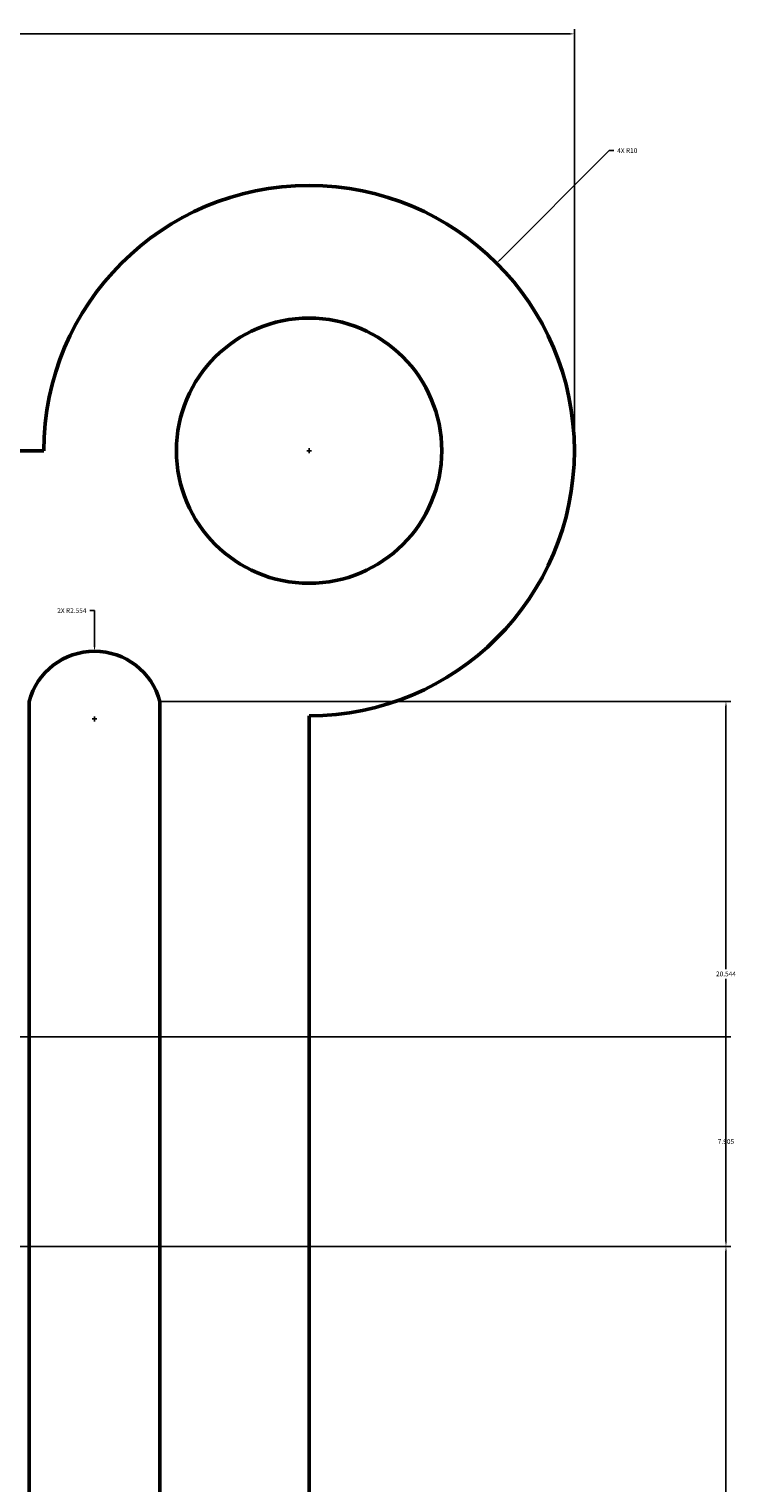
# Model space of a CAD drawing. Units: inches. Extents: x -14 to 108, y -9 to 83.
# Tile 13 of 13: x 82 to 108, y 28 to 83. Entities that reach past the tile are written whole.
import ezdxf

# ---------------------------------------------------------------- set-up
doc = ezdxf.new("R2010")
doc.units = ezdxf.units.IN
doc.header["$MEASUREMENT"] = 0
doc.layers.add('M-DIMS', color=2, linetype='Continuous', lineweight=18)
doc.layers.add('M-OUTL', color=7, linetype='Continuous', lineweight=50)
doc.styles.get("Standard").update_dxf_attribs({"font": 'arial.ttf'})
doc.dimstyles.get("Standard").update_dxf_attribs({"dimtxt": 0.18, "dimasz": 0.18, "dimexe": 0.18, "dimexo": 0.0625, "dimgap": 0.09, "dimtad": 0, "dimtih": 1, "dimtoh": 1, "dimzin": 0, "dimdsep": 46, "dimtxsty": 'Standard', "dimcen": 0.09, "dimadec": 0, "dimazin": 0, "dimtfac": 1, "dimtofl": 0, "dimtmove": 0, "dimatfit": 3, "dimfxl": 1, "dimtolj": 1, "dimtzin": 0, "dimarcsym": 0})

# ---------------------------------------------------------------- blocks, each defined once
blk = doc.blocks.new('SLOT-VERTICAL')
for points in [[(0, 1.021), (0, 40.458)], [(4.933, 40.458), (4.933, 1.021)]]:
    blk.add_lwpolyline(points)
for centre, radius, start, end in [((2.466, 39.797), 2.554, 15, 165), ((2.466, 3.488), 3.489, 225, 315)]:
    blk.add_arc(centre, radius, start, end)
blk = doc.blocks.new('HOLE-D10')
blk.add_circle((5, 5), 5)
blk = doc.blocks.new('*D4')
at = {"layer": 'Defpoints', "color": 0, "transparency": 16777216}
for p in [(102.098, 82.834), (-7.902, 67.119), (102.098, 67.119)]:
    blk.add_point(p, dxfattribs=at)
at = {"layer": 'M-DIMS', "color": 0, "lineweight": -2, "transparency": 16777216}
for p, q in [((-7.902, 67.182), (-7.902, 83.014)), ((-7.722, 82.834), (46.818, 82.834)), ((101.918, 82.834), (47.378, 82.834)), ((102.098, 67.182), (102.098, 83.014))]:
    blk.add_line(p, q, dxfattribs=at)
at = {"layer": 'M-DIMS', "color": 0, "transparency": 16777216}
for points in [[(-7.722, 82.864), (-7.722, 82.804), (-7.902, 82.834)], [(101.918, 82.864), (101.918, 82.804), (102.098, 82.834)]]:
    blk.add_solid(points, dxfattribs=at)
at = {"layer": 'M-DIMS', "color": 0, "transparency": 16777216, "insert": (47.098, 82.834), "char_height": 0.18, "attachment_point": 5}
blk.add_mtext('\\A1;110', dxfattribs=at)
blk = doc.blocks.new('*D11')
at = {"layer": 'Defpoints', "color": 0, "transparency": 16777216}
for p in [(47.098, 37.119), (107.813, 37.119), (86.478, 18.227)]:
    blk.add_point(p, dxfattribs=at)
at = {"layer": 'M-DIMS', "color": 0, "lineweight": -2, "transparency": 16777216}
for p, q in [((47.16, 37.119), (107.993, 37.119)), ((107.813, 36.939), (107.813, 27.855)), ((107.813, 18.407), (107.813, 27.491)), ((86.541, 18.227), (107.993, 18.227))]:
    blk.add_line(p, q, dxfattribs=at)
at = {"layer": 'M-DIMS', "color": 0, "transparency": 16777216}
for points in [[(107.783, 36.939), (107.843, 36.939), (107.813, 37.119)], [(107.783, 18.407), (107.843, 18.407), (107.813, 18.227)]]:
    blk.add_solid(points, dxfattribs=at)
at = {"layer": 'M-DIMS', "color": 0, "transparency": 16777216, "insert": (107.813, 27.673), "char_height": 0.18, "attachment_point": 5}
blk.add_mtext('\\A1;18.892', dxfattribs=at)
blk = doc.blocks.new('*D12')
at = {"layer": 'Defpoints', "color": 0, "transparency": 16777216}
for p in [(86.478, 57.664), (107.813, 57.664), (47.098, 37.119)]:
    blk.add_point(p, dxfattribs=at)
at = {"layer": 'M-DIMS', "color": 0, "lineweight": -2, "transparency": 16777216}
for p, q in [((86.541, 57.664), (107.993, 57.664)), ((107.813, 57.484), (107.813, 47.573)), ((107.813, 37.299), (107.813, 47.21)), ((47.16, 37.119), (107.993, 37.119))]:
    blk.add_line(p, q, dxfattribs=at)
at = {"layer": 'M-DIMS', "color": 0, "transparency": 16777216}
for points in [[(107.783, 57.484), (107.843, 57.484), (107.813, 57.664)], [(107.783, 37.299), (107.843, 37.299), (107.813, 37.119)]]:
    blk.add_solid(points, dxfattribs=at)
at = {"layer": 'M-DIMS', "color": 0, "transparency": 16777216, "insert": (107.813, 47.392), "char_height": 0.18, "attachment_point": 5}
blk.add_mtext('\\A1;20.544', dxfattribs=at)
blk = doc.blocks.new('*D21')
at = {"layer": 'Defpoints', "color": 0, "transparency": 16777216}
for p in [(65.47, 45.024), (107.813, 45.024), (47.098, 37.119)]:
    blk.add_point(p, dxfattribs=at)
at = {"layer": 'M-DIMS', "color": 0, "lineweight": -2, "transparency": 16777216}
for p, q in [((65.532, 45.024), (107.993, 45.024)), ((107.813, 44.844), (107.813, 41.254)), ((107.813, 37.299), (107.813, 40.89)), ((47.16, 37.119), (107.993, 37.119))]:
    blk.add_line(p, q, dxfattribs=at)
at = {"layer": 'M-DIMS', "color": 0, "transparency": 16777216}
for points in [[(107.783, 44.844), (107.843, 44.844), (107.813, 45.024)], [(107.783, 37.299), (107.843, 37.299), (107.813, 37.119)]]:
    blk.add_solid(points, dxfattribs=at)
at = {"layer": 'M-DIMS', "color": 0, "transparency": 16777216, "insert": (107.813, 41.072), "char_height": 0.18, "attachment_point": 5}
blk.add_mtext('\\A1;7.905', dxfattribs=at)
blk = doc.blocks.new('*D24')
at = {"layer": 'Defpoints', "color": 0, "transparency": 16777216}
for p in [(99.169, 74.19), (92.098, 67.119)]:
    blk.add_point(p, dxfattribs=at)
at = {"layer": 'M-DIMS', "color": 0, "lineweight": -2, "transparency": 16777216}
for p, q in [((103.412, 78.433), (99.296, 74.317)), ((103.592, 78.433), (103.412, 78.433)), ((92.008, 67.119), (92.188, 67.119)), ((92.098, 67.029), (92.098, 67.209))]:
    blk.add_line(p, q, dxfattribs=at)
at = {"layer": 'M-DIMS', "color": 0, "transparency": 16777216}
blk.add_solid([(99.275, 74.339), (99.318, 74.296), (99.169, 74.19)], dxfattribs=at)
at = {"layer": 'M-DIMS', "color": 0, "transparency": 16777216, "insert": (104.094, 78.433), "char_height": 0.18, "attachment_point": 5}
blk.add_mtext('\\A1;4X R10', dxfattribs=at)
blk = doc.blocks.new('*D27')
at = {"layer": 'Defpoints', "color": 0, "transparency": 16777216}
for p in [(84.011, 59.557), (84.011, 57.003)]:
    blk.add_point(p, dxfattribs=at)
at = {"layer": 'M-DIMS', "color": 0, "lineweight": -2, "transparency": 16777216}
for p, q in [((83.831, 61.089), (84.011, 61.089)), ((84.011, 61.089), (84.011, 59.737)), ((84.011, 56.913), (84.011, 57.093)), ((83.921, 57.003), (84.101, 57.003))]:
    blk.add_line(p, q, dxfattribs=at)
at = {"layer": 'M-DIMS', "color": 0, "transparency": 16777216}
blk.add_solid([(84.041, 59.737), (83.981, 59.737), (84.011, 59.557)], dxfattribs=at)
at = {"layer": 'M-DIMS', "color": 0, "transparency": 16777216, "insert": (83.156, 61.089), "char_height": 0.18, "attachment_point": 5}
blk.add_mtext('\\A1;2X R2.554', dxfattribs=at)

msp = doc.modelspace()

# ---------------------------------------------------------------- linework, layer by layer
at = {"layer": 'M-OUTL'}
for points in [[(82.0979, 67.1193), (12.0979, 67.1193)], [(92.0979, 17.1193), (92.0979, 57.1193)]]:
    msp.add_lwpolyline(points, dxfattribs=at)
msp.add_arc((92.0979, 67.1193), 10, 270, 180, dxfattribs=at)

# ---------------------------------------------------------------- block references
for name, p in [('HOLE-D10', (87.098, 62.119)), ('SLOT-VERTICAL', (81.545, 17.206))]:
    msp.add_blockref(name, p, dxfattribs=at)

# ---------------------------------------------------------------- dimensions: what is measured, and where the dimension line sits
at = {"layer": 'M-DIMS'}
dim = msp.add_linear_dim(base=(102.0979, 82.8343), p1=(-7.9021, 67.1193), p2=(102.0979, 67.1193), dimstyle='Standard', override={"dimdec": 0, "dimlfac": 1, "dimrnd": 0, "dimzin": 0, "dimdsep": 46, "dimlunit": 2}, dxfattribs=at)
dim.commit()
dim.dimension.update_dxf_attribs({"geometry": '*D4', "text_midpoint": (47.0979, 82.8343)})
for center, mpoint, text, override, picture, middle in [((92.0979, 67.1193), (99.1692, 74.1902), '4X <>', {"dimdec": 0, "dimlfac": 1, "dimrnd": 0, "dimzin": 0, "dimdsep": 46, "dimlunit": 2}, '*D24', (104.0937, 78.4327)), ((84.0115, 57.0027), (84.011, 59.5566), '2X <>', {"dimdec": 3, "dimlfac": 1, "dimrnd": 0, "dimzin": 0, "dimdsep": 46, "dimlunit": 2}, '*D27', (83.1563, 61.0889))]:
    dim = msp.add_radius_dim(center=center, mpoint=mpoint, text=text, dimstyle='Standard', override=override, dxfattribs=at)
    dim.commit()
    dim.dimension.update_dxf_attribs({"geometry": picture, "text_midpoint": middle, "dimtype": 164})
for base, p1, p2, picture, middle in [((107.8129, 57.6637), (47.0979, 37.1193), (86.4784, 57.6637), '*D12', (107.8129, 47.3915)), ((107.8129, 45.0241), (47.0979, 37.1193), (65.4695, 45.0241), '*D21', (107.8129, 41.0717)), ((107.8129, 37.1193), (86.4784, 18.2274), (47.0979, 37.1193), '*D11', (107.8129, 27.6733))]:
    dim = msp.add_linear_dim(base=base, p1=p1, p2=p2, angle=90, dimstyle='Standard', override={"dimdec": 3, "dimlfac": 1, "dimrnd": 0, "dimzin": 0, "dimdsep": 46, "dimlunit": 2}, dxfattribs=at)
    dim.commit()
    dim.dimension.update_dxf_attribs({"geometry": picture, "text_midpoint": middle})

doc.saveas('drawing.dxf')
